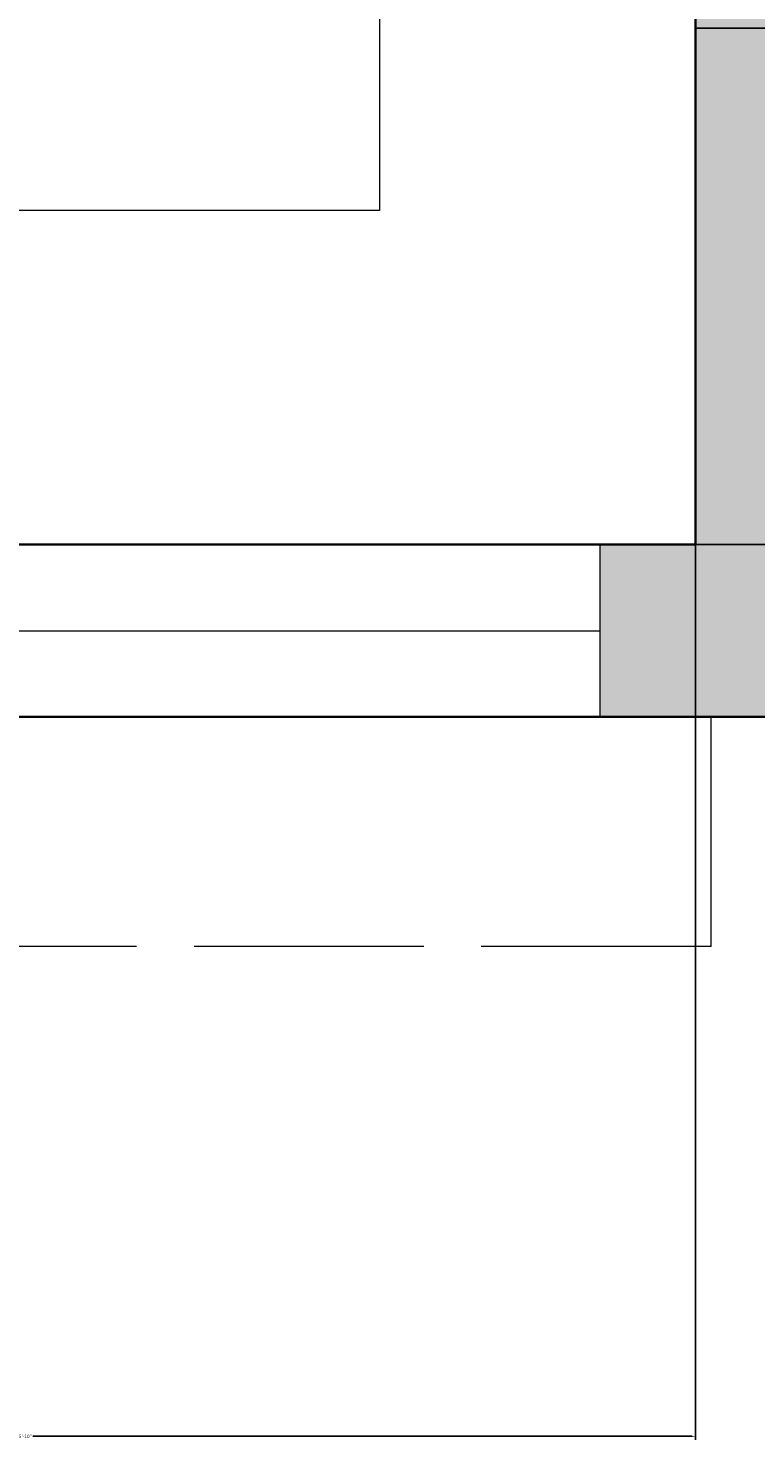
# Model space of a CAD drawing. Units: inches. Extents: x -5 to 482, y -460 to 66.
# Tile 11 of 31: x 180 to 218, y -460 to -386. Entities that reach past the tile are written whole.
import ezdxf

# ---------------------------------------------------------------- set-up
doc = ezdxf.new("R2010")
doc.units = ezdxf.units.IN
doc.header["$MEASUREMENT"] = 0
doc.linetypes.add('ACAD_ISO02W100', pattern=[15, 12, -3])
for name, color, linetype, lineweight in [('A-ANNO-DIMS', 2, 'Continuous', 18), ('A-ANNO-SYMB', 7, 'Continuous', 18), ('A-GLAZ', 4, 'Continuous', 18), ('A-GLAZ-OVHD', 4, 'ACAD_ISO02W100', 13), ('A-WALL', 7, 'Continuous', 35), ('A-WALL-PATT', 152, 'Continuous', 13)]:
    doc.layers.add(name, color=color, linetype=linetype, lineweight=lineweight)
doc.styles.get("Standard").update_dxf_attribs({"font": 'arial.ttf'})
doc.dimstyles.get("Standard").update_dxf_attribs({"dimtxt": 0.18, "dimasz": 0.18, "dimexe": 0.18, "dimexo": 0.0625, "dimgap": 0.09, "dimtad": 0, "dimtih": 1, "dimtoh": 1, "dimdec": 0, "dimzin": 0, "dimdsep": 46, "dimlunit": 3, "dimtxsty": 'Standard', "dimcen": 0.09, "dimadec": 0, "dimazin": 0, "dimtfac": 1, "dimtdec": 0, "dimtofl": 0, "dimtmove": 0, "dimatfit": 3, "dimfxl": 1, "dimtolj": 1, "dimtzin": 0, "dimarcsym": 0})

# ---------------------------------------------------------------- blocks, each defined once
blk = doc.blocks.new('WIN-GLAZ-60IN')
for p, q in [((0, 9), (60, 9)), ((0, 4.5), (60, 4.5)), ((60, 0), (0, 0))]:
    blk.add_line(p, q)
blk = doc.blocks.new('WIN-SHADE-72IN')
for p, q in [((0, 12), (72, 12)), ((0, 12), (0, 0)), ((72, 12), (72, 0))]:
    blk.add_line(p, q)
blk = doc.blocks.new('*D71')
at = {"layer": 'A-ANNO-DIMS', "color": 0, "lineweight": -2, "transparency": 16777216}
for p, q in [((144.377, -385.924), (144.377, -459.629)), ((214.377, -385.924), (214.377, -459.629)), ((144.557, -459.449), (178.978, -459.449)), ((214.197, -459.449), (179.776, -459.449))]:
    blk.add_line(p, q, dxfattribs=at)
at = {"layer": 'A-ANNO-DIMS', "color": 0, "transparency": 16777216}
for points in [[(144.557, -459.419), (144.557, -459.479), (144.377, -459.449)], [(214.197, -459.419), (214.197, -459.479), (214.377, -459.449)]]:
    blk.add_solid(points, dxfattribs=at)
at = {"layer": 'Defpoints', "color": 0, "transparency": 16777216}
for p in [(144.377, -385.861), (214.377, -385.861), (214.377, -459.449)]:
    blk.add_point(p, dxfattribs=at)
at = {"layer": 'A-ANNO-DIMS', "color": 0, "transparency": 16777216, "insert": (179.377, -459.449), "char_height": 0.18, "attachment_point": 5}
blk.add_mtext('\\A1;5\'-10"', dxfattribs=at)
blk = doc.blocks.new('*D74')
at = {"layer": 'A-ANNO-DIMS', "color": 0, "lineweight": -2, "transparency": 16777216}
for p, q in [((214.439, -295.861), (468.157, -295.861)), ((467.977, -296.041), (467.977, -340.679)), ((467.977, -385.681), (467.977, -341.043)), ((214.439, -385.861), (468.157, -385.861))]:
    blk.add_line(p, q, dxfattribs=at)
at = {"layer": 'A-ANNO-DIMS', "color": 0, "transparency": 16777216}
for points in [[(467.947, -296.041), (468.007, -296.041), (467.977, -295.861)], [(467.947, -385.681), (468.007, -385.681), (467.977, -385.861)]]:
    blk.add_solid(points, dxfattribs=at)
at = {"layer": 'Defpoints', "color": 0, "transparency": 16777216}
for p in [(214.377, -295.861), (467.977, -295.861), (214.377, -385.861)]:
    blk.add_point(p, dxfattribs=at)
at = {"layer": 'A-ANNO-DIMS', "color": 0, "transparency": 16777216, "insert": (467.977, -340.861), "char_height": 0.18, "attachment_point": 5}
blk.add_mtext('\\A1;7\'-6"', dxfattribs=at)
blk = doc.blocks.new('*D75')
at = {"layer": 'A-ANNO-DIMS', "color": 0, "lineweight": -2, "transparency": 16777216}
for p, q in [((214.439, -385.861), (468.157, -385.861)), ((467.977, -386.041), (467.977, -399.173)), ((467.977, -412.669), (467.977, -399.537)), ((214.439, -412.849), (468.157, -412.849))]:
    blk.add_line(p, q, dxfattribs=at)
at = {"layer": 'A-ANNO-DIMS', "color": 0, "transparency": 16777216}
for points in [[(467.947, -386.041), (468.007, -386.041), (467.977, -385.861)], [(467.947, -412.669), (468.007, -412.669), (467.977, -412.849)]]:
    blk.add_solid(points, dxfattribs=at)
at = {"layer": 'Defpoints', "color": 0, "transparency": 16777216}
for p in [(214.377, -385.861), (467.977, -385.861), (214.377, -412.849)]:
    blk.add_point(p, dxfattribs=at)
at = {"layer": 'A-ANNO-DIMS', "color": 0, "transparency": 16777216, "insert": (467.977, -399.355), "char_height": 0.18, "attachment_point": 5}
blk.add_mtext('\\A1;2\'-3"', dxfattribs=at)

msp = doc.modelspace()

# ---------------------------------------------------------------- hatches: boundary and pattern name
at = {"layer": 'A-WALL-PATT'}
h = msp.add_hatch(color=256, dxfattribs=at)
h.dxf.hatch_style = 1
h.paths.add_polyline_path([(149.377, -412.849), (144.377, -412.849), (144.377, -283.849), (144.377, -279.349), (133.877, -279.349), (133.877, -283.849), (139.877, -283.849), (139.877, -412.849), (133.51, -412.849), (133.51, -413.916), (102.652, -413.916), (102.652, -421.02), (133.51, -421.02), (133.51, -421.849), (149.377, -421.849)])
h.paths.add_polyline_path([(226.054, -412.849), (218.877, -412.849), (218.877, -350.849), (262.877, -350.849), (262.877, -386.849), (267.377, -386.849), (267.377, -283.849), (270.377, -283.849), (270.377, -279.349), (244.877, -279.349), (244.877, -283.849), (262.877, -283.849), (262.877, -346.349), (218.877, -346.349), (218.877, -283.849), (220.877, -283.849), (220.877, -279.349), (214.377, -279.349), (214.377, -283.849), (214.377, -412.849), (209.377, -412.849), (209.377, -421.849), (226.054, -421.849)])
h.paths.add_polyline_path([(315.815, -412.849), (250.054, -412.849), (250.054, -421.849), (315.815, -421.849)])
h.paths.add_polyline_path([(430.377, -378.349), (421.377, -378.349), (421.377, -412.849), (375.815, -412.849), (375.815, -421.849), (430.377, -421.849)])
h.paths.add_polyline_path([(78.691, -413.916), (47.68, -413.916), (47.68, -412.849), (41.877, -412.849), (41.877, -283.849), (109.877, -283.849), (109.877, -279.349), (41.877, -279.349), (41.877, -241.849), (32.877, -241.849), (32.877, -421.849), (47.68, -421.849), (47.68, -421.02), (78.691, -421.02)])
h.paths.add_polyline_path([(41.877, -144.349), (154.377, -144.349), (154.377, -137.849), (149.877, -137.849), (149.877, -139.849), (41.877, -139.849), (41.877, -97.849), (32.877, -97.849), (32.877, -181.849), (41.877, -181.849)])
h.paths.add_polyline_path([(430.377, -241.849), (421.377, -241.849), (421.377, -279.349), (309.377, -279.349), (309.377, -170.349), (304.877, -170.349), (304.877, -279.349), (294.377, -279.349), (294.377, -283.849), (421.377, -283.849), (421.377, -318.349), (430.377, -318.349)])
h.paths.add_polyline_path([(430.377, -119.849), (421.377, -119.849), (421.377, -139.849), (419.377, -139.849), (419.377, -144.349), (421.377, -144.349), (421.377, -181.849), (430.377, -181.849)])
h.paths.add_polyline_path([(395.377, -139.849), (377.377, -139.849), (377.377, -75.849), (421.377, -75.849), (421.377, -95.849), (430.377, -95.849), (430.377, -45.599), (421.377, -45.599), (421.377, -71.349), (377.377, -71.349), (377.377, -22.849), (372.877, -22.849), (372.877, -139.849), (242.877, -139.849), (242.877, -137.849), (238.377, -137.849), (238.377, -144.349), (304.877, -144.349), (304.877, -146.349), (309.377, -146.349), (309.377, -144.349), (395.377, -144.349)])
h.paths.add_polyline_path([(65.877, 13.151), (32.877, 13.151), (32.877, -37.849), (41.877, -37.849), (41.877, 4.151), (65.877, 4.151)])
h.paths.add_polyline_path([(166.377, 13.151), (125.877, 13.151), (125.877, 4.151), (149.877, 4.151), (149.877, -113.849), (154.377, -113.849), (154.377, 4.151), (166.377, 4.151)])
h.paths.add_polyline_path([(277.877, 13.151), (226.377, 13.151), (226.377, 4.151), (238.377, 4.151), (238.377, -113.849), (242.877, -113.849), (242.877, 4.151), (277.877, 4.151)])
h.paths.add_polyline_path([(430.377, 13.151), (337.877, 13.151), (337.877, 4.151), (372.877, 4.151), (372.877, 1.151), (377.377, 1.151), (377.377, 4.151), (421.377, 4.151), (421.377, -21.599), (430.377, -21.599)])

# ---------------------------------------------------------------- linework, layer by layer
at = {"layer": 'A-ANNO-SYMB'}
for p, q in [((197.881, -295.861), (197.881, -395.385)), ((197.881, -395.385), (162.322, -395.385))]:
    msp.add_line(p, q, dxfattribs=at)
at = {"layer": 'A-GLAZ'}
msp.add_line((209.377, -412.849), (209.377, -421.849), dxfattribs=at)
at = {"layer": 'A-WALL'}
for p, q in [((214.377, -283.849), (214.377, -412.849)), ((144.377, -412.849), (214.377, -412.849)), ((133.51, -421.849), (430.377, -421.849))]:
    msp.add_line(p, q, dxfattribs=at)

# ---------------------------------------------------------------- block references
at = {"layer": 'A-GLAZ'}
msp.add_blockref('WIN-GLAZ-60IN', (149.377, -421.849), dxfattribs=at)
at = {"layer": 'A-GLAZ-OVHD', "rotation": 180}
msp.add_blockref('WIN-SHADE-72IN', (215.191, -421.848), dxfattribs=at)

# ---------------------------------------------------------------- dimensions: what is measured, and where the dimension line sits
at = {"layer": 'A-ANNO-DIMS'}
for base, p1, p2, picture, middle in [((467.977, -295.861), (214.377, -385.861), (214.377, -295.861), '*D74', (467.977, -340.861)), ((467.977, -385.861), (214.377, -412.849), (214.377, -385.861), '*D75', (467.977, -399.355))]:
    dim = msp.add_linear_dim(base=base, p1=p1, p2=p2, angle=90, dimstyle='Standard', override={"dimdec": 1, "dimlfac": 1, "dimrnd": 0, "dimzin": 1, "dimdsep": 46, "dimlunit": 4, "dimfrac": 2}, dxfattribs=at)
    dim.commit()
    dim.dimension.update_dxf_attribs({"geometry": picture, "text_midpoint": middle})
dim = msp.add_linear_dim(base=(214.377, -459.449), p1=(144.377, -385.861), p2=(214.377, -385.861), dimstyle='Standard', override={"dimdec": 1, "dimlfac": 1, "dimrnd": 0, "dimzin": 1, "dimdsep": 46, "dimlunit": 4, "dimfrac": 2}, dxfattribs=at)
dim.commit()
dim.dimension.update_dxf_attribs({"geometry": '*D71', "text_midpoint": (179.377, -459.449)})

doc.saveas('drawing.dxf')
